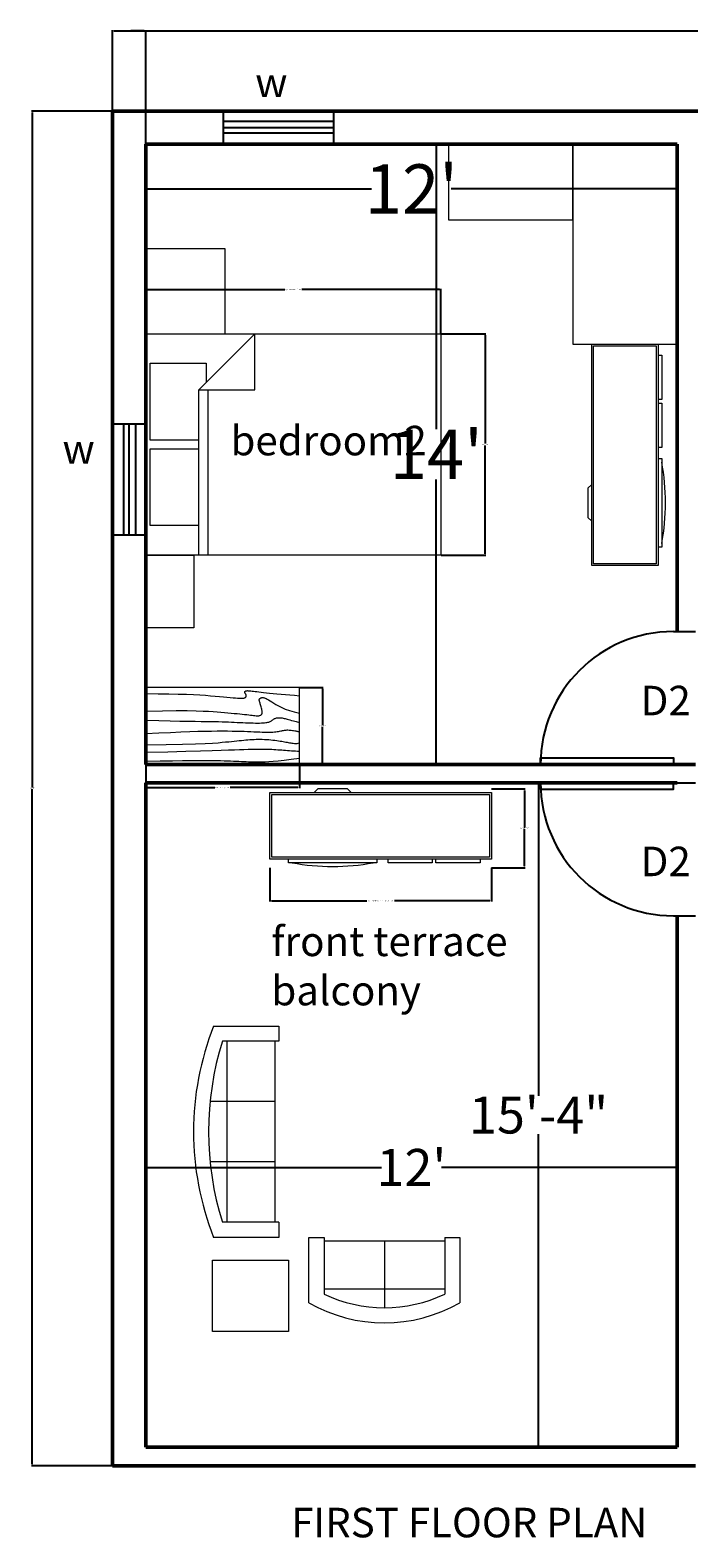
# Model space of a CAD drawing. Units: inches. Extents: x -10 to 557, y -66 to 886.
# Tile 4 of 6: x 31 to 210, y 478 to 886. Entities that reach past the tile are written whole.
import ezdxf

# ---------------------------------------------------------------- set-up
doc = ezdxf.new("R2010")
doc.units = ezdxf.units.IN
doc.header["$MEASUREMENT"] = 0
for name, color, linetype, lineweight in [('A-ANNO-DIMS', 2, 'Continuous', 18), ('A-ANNO-TEXT', 7, 'Continuous', 18), ('A-AREA-IDEN', 7, 'Continuous', 25), ('A-DOOR', 4, 'Continuous', 25), ('A-FURN', 8, 'Continuous', 18), ('A-GLAZ', 4, 'Continuous', 25), ('A-WALL', 7, 'Continuous', 50)]:
    doc.layers.add(name, color=color, linetype=linetype, lineweight=lineweight)
doc.styles.get("Standard").update_dxf_attribs({"font": 'arial.ttf'})
doc.dimstyles.get("Standard").update_dxf_attribs({"dimtxt": 0.3, "dimasz": 0.4, "dimexe": 0.18, "dimexo": 0.0625, "dimgap": 0.09, "dimtad": 0, "dimtih": 1, "dimtoh": 1, "dimdec": 0, "dimrnd": 8, "dimzin": 0, "dimdsep": 46, "dimlunit": 3, "dimtxsty": 'Standard', "dimcen": 0.09, "dimadec": 0, "dimazin": 0, "dimtfac": 1, "dimtdec": 0, "dimtofl": 0, "dimtmove": 0, "dimatfit": 3, "dimfxl": 1, "dimtolj": 1, "dimtzin": 0, "dimarcsym": 0})

# ---------------------------------------------------------------- blocks, each defined once
blk = doc.blocks.new('*U2')
for p, q in [((0, 0), (0, -6)), ((36, 0), (36, -6))]:
    blk.add_line(p, q)
blk.add_lwpolyline([(0, 0), (0, 36), (1.75, 36), (1.75, 0)], close=True)
blk.add_arc((0, 0), 36, 0, 90)
blk = doc.blocks.new('*U5')
for p, q in [((0, 0), (0, -6)), ((-36, 0), (-36, -6))]:
    blk.add_line(p, q)
blk.add_lwpolyline([(0, 0), (0, 36), (-1.75, 36), (-1.75, 0)], close=True)
blk.add_arc((0, 0), 36, 90, 180)
blk = doc.blocks.new('Entertainment Center')
for p, q in [((-4, 0), (-5, -1)), ((4, 0), (-4, 0)), ((5, -1), (4, 0)), ((-17, -19), (-17, -1)), ((-17, -1), (43, -1)), ((-16.5, -18.5), (-16.5, -1.5)), ((-16.5, -1.5), (42.5, -1.5)), ((42.5, -1.5), (42.5, -18.5)), ((43, -1), (43, -19)), ((43, -19), (-17, -19)), ((42.5, -18.5), (-16.5, -18.5)), ((-12, -20), (-12, -19)), ((12, -20), (-12, -20)), ((12, -19), (12, -20)), ((15, -20), (15, -19)), ((27, -20), (15, -20)), ((27, -19), (27, -20)), ((28, -20), (28, -19)), ((40, -20), (28, -20)), ((40, -19), (40, -20))]:
    blk.add_line(p, q)
blk.add_arc((0, 40), 61, 259.6111, 280.3889)
blk = doc.blocks.new('Sofa - Roundback 7 ft.')
for p, q in [((-36.000027, -34), (-36.000027, -11.4696)), ((-12.00002, -32.4421), (-12.00003, -6.5971)), ((11.99997, -32.4421), (11.99998, -6.5971)), ((35.99998, -34), (35.99998, -11.4696)), ((-35.999844, -13.3819), (35.9998, -13.3819)), ((-36.000027, -32.4421), (35.99998, -32.4421))]:
    blk.add_line(p, q)
for points in [[(-36.000027, -34), (-42.000027, -34), (-42.000027, -8)], [(41.99998, -8), (41.99998, -34), (35.99998, -34)]]:
    blk.add_lwpolyline(points)
for centre, radius, start, end in [((0, -114.25), 114.25, 68.43141, 111.5686), ((-0.00001, -127.1968), 121.1968, 72.72033, 107.2797)]:
    blk.add_arc(centre, radius, start, end)
blk = doc.blocks.new('Sofa - Roundback Loveseat 5 ft.')
for p, q in [((-24, -33.99998), (-24, -11.46958)), ((0, -32.44198), (0, -5.99998)), ((24.00004, -33.99998), (24.00004, -11.46958)), ((-23.9998, -13.38178), (23.99986, -13.38178)), ((-24, -32.44198), (24.00004, -32.44198))]:
    blk.add_line(p, q)
for points in [[(-24, -33.99998), (-30, -33.99998), (-30, -7.99998)], [(30.00004, -7.99998), (30.00004, -33.99998), (24.00004, -33.99998)]]:
    blk.add_lwpolyline(points)
for centre, radius, start, end in [((0, -60.24998), 60.24998, 60.13715, 119.8628), ((0, -61.38438), 55.38444, 64.32083, 115.6792)]:
    blk.add_arc(centre, radius, start, end)
blk = doc.blocks.new('Bed - Queen')
for p, q in [((0, -80.00003), (0, 0)), ((0, 0), (59.99999, 0)), ((59.99999, 0), (59.99999, -80.00003)), ((7.99999, -1.2), (28.79998, -1.2)), ((7.99999, -14.4), (7.99999, -1.2)), ((28.79998, -1.2), (28.79998, -14.4)), ((31.19999, -1.2), (51.99999, -1.2)), ((31.19999, -14.4), (31.19999, -1.2)), ((51.99999, -1.2), (51.99999, -16.4)), ((0, -14.4), (44.8, -14.4)), ((59.99999, -29.6), (44.8, -14.4)), ((44.8, -14.4), (44.8, -29.6)), ((44.8, -16.8), (0, -16.8)), ((51.99999, -16.4), (46.79936, -16.4)), ((44.8, -29.6), (59.99999, -29.6)), ((59.99999, -80.00003), (0, -80.00003))]:
    blk.add_line(p, q)
blk = doc.blocks.new('Table - Rectangular Woodgrain 60 x 30 in.')
for p, q in [((0, 0), (0, -30)), ((60, 0), (0, 0)), ((60, -30), (60, 0)), ((0, -30), (60, -30))]:
    blk.add_line(p, q)
for points in [[(0, -2.4), (4.8155, -2.418), (9.0302, -2.4688), (12.709, -2.5477), (15.9167, -2.65), (18.7181, -2.7711), (21.1781, -2.9063), (23.3616, -3.0508), (25.3333, -3.2), (27.1477, -3.3495), (28.8172, -3.4958), (30.3437, -3.636), (31.7291, -3.7667), (32.9756, -3.8849), (34.0849, -3.9875), (35.059, -4.0714), (35.9, -4.1334), (36.6114, -4.1711), (37.2041, -4.1854), (37.6906, -4.1779), (38.0833, -4.15), (38.3948, -4.1034), (38.6375, -4.0396), (38.8239, -3.9602), (38.9666, -3.8667), (39.0764, -3.7608), (39.1573, -3.6448), (39.2116, -3.521), (39.2416, -3.3917), (39.2498, -3.2593), (39.2385, -3.1261), (39.21, -2.9944), (39.1666, -2.8667), (39.111, -2.7447), (39.0468, -2.6281), (38.978, -2.5163), (38.9083, -2.4083), (38.8418, -2.3035), (38.7823, -2.201), (38.7337, -2.1001), (38.7, -2), (38.6844, -1.9003), (38.6875, -1.8021), (38.7094, -1.707), (38.75, -1.6167), (38.8094, -1.5326), (38.8875, -1.4563), (38.9844, -1.3893), (39.1, -1.3333), (39.2351, -1.2896), (39.3937, -1.2583), (39.5804, -1.2396), (39.8, -1.2333), (40.057, -1.2396), (40.3562, -1.2583), (40.7023, -1.2896), (41.1, -1.3333), (41.5547, -1.3895), (42.0755, -1.4573), (42.6721, -1.5361), (43.3542, -1.625), (44.1316, -1.7233), (45.014, -1.8302), (46.0114, -1.9449), (47.1333, -2.0667), (48.3862, -2.1947), (49.7625, -2.3281), (51.2513, -2.4663), (52.8416, -2.6083), (54.5226, -2.7535), (56.2833, -2.9011), (58.1127, -3.0501), (60, -3.2)], [(0, -9.2), (6.5759, -9.0858), (11.9385, -9.0365), (16.2527, -9.0418), (19.6833, -9.0917), (22.3952, -9.1759), (24.5531, -9.2844), (26.322, -9.4069), (27.8666, -9.5333), (29.3241, -9.6553), (30.7203, -9.7719), (32.0532, -9.8837), (33.3208, -9.9917), (34.5213, -10.0965), (35.6526, -10.199), (36.7128, -10.2999), (37.7, -10.4), (38.6129, -10.4996), (39.4531, -10.5969), (40.223, -10.6895), (40.925, -10.775), (41.5613, -10.8512), (42.1344, -10.9156), (42.6465, -10.966), (43.1, -11), (43.4976, -11.0158), (43.8437, -11.0136), (44.143, -10.9942), (44.4, -10.9583), (44.6195, -10.9069), (44.8062, -10.8406), (44.9648, -10.7603), (45.1, -10.6667), (45.2155, -10.5598), (45.3114, -10.4365), (45.3871, -10.2929), (45.4416, -10.125), (45.4743, -9.929), (45.4844, -9.7011), (45.4709, -9.4371), (45.4333, -9.1333), (45.3716, -8.7883), (45.2896, -8.4104), (45.1919, -8.0107), (45.0833, -7.6), (44.9685, -7.1893), (44.8521, -6.7896), (44.7388, -6.4117), (44.6333, -6.0667), (44.54, -5.7628), (44.4614, -5.4979), (44.4001, -5.2675), (44.3583, -5.0667), (44.3384, -4.8909), (44.3427, -4.7354), (44.3736, -4.5956), (44.4333, -4.4667), (44.5236, -4.3453), (44.6427, -4.2333), (44.7884, -4.1339), (44.9583, -4.05), (45.1501, -3.9849), (45.3614, -3.9417), (45.59, -3.9234), (45.8333, -3.9333), (46.0915, -3.9749), (46.3734, -4.0531), (46.6906, -4.1736), (47.0542, -4.3417), (47.4756, -4.5629), (47.9661, -4.8427), (48.5372, -5.1866), (49.2, -5.6), (49.9676, -6.0844), (50.8594, -6.625), (51.8965, -7.2031), (53.1, -7.8), (54.491, -8.3969), (56.0906, -8.975), (57.9199, -9.5156), (60, -10)], [(0, -12.8), (5.1847, -12.9322), (9.6213, -13.0323), (13.3963, -13.1059), (16.5958, -13.1583), (19.3063, -13.1952), (21.614, -13.2219), (23.6054, -13.2439), (25.3666, -13.2667), (26.9728, -13.2947), (28.4531, -13.3281), (29.8256, -13.3663), (31.1083, -13.4083), (32.3191, -13.4535), (33.476, -13.501), (34.597, -13.5501), (35.7, -13.6), (36.7984, -13.6497), (37.8875, -13.6979), (38.9578, -13.743), (40, -13.7833), (41.0047, -13.8174), (41.9625, -13.8438), (42.864, -13.8607), (43.7, -13.8667), (44.4631, -13.8604), (45.1552, -13.8417), (45.7801, -13.8104), (46.3416, -13.7667), (46.8439, -13.7104), (47.2906, -13.6417), (47.6858, -13.5604), (48.0333, -13.4667), (48.3375, -13.3608), (48.6042, -13.2448), (48.8396, -13.121), (49.05, -12.9917), (49.2417, -12.8593), (49.4208, -12.7261), (49.5937, -12.5944), (49.7667, -12.4667), (49.9452, -12.3451), (50.1323, -12.2313), (50.3303, -12.1268), (50.5416, -12.0333), (50.7686, -11.9524), (51.0135, -11.8854), (51.2788, -11.8341), (51.5666, -11.8), (51.8785, -11.7843), (52.2116, -11.7865), (52.562, -11.8059), (52.926, -11.8417), (53.2998, -11.8931), (53.6795, -11.9594), (54.0614, -12.0397), (54.4416, -12.1333), (54.8223, -12.2401), (55.2293, -12.3625), (55.6942, -12.5037), (56.2489, -12.6667), (56.9251, -12.8547), (57.7545, -13.0708), (58.7689, -13.3182), (60, -13.6)], [(0, -18), (5.124, -17.7273), (9.6609, -17.5057), (13.6705, -17.3303), (17.2125, -17.1958), (20.3467, -17.0973), (23.1328, -17.0297), (25.6307, -16.9878), (27.9, -16.9667), (29.9928, -16.9617), (31.9302, -16.9703), (33.7254, -16.9907), (35.3917, -17.0208), (36.9423, -17.0588), (38.3906, -17.1026), (39.7499, -17.1503), (41.0333, -17.2), (42.2519, -17.2496), (43.4073, -17.2969), (44.4986, -17.3395), (45.525, -17.375), (46.4858, -17.4012), (47.3802, -17.4156), (48.2074, -17.416), (48.9667, -17.4), (49.6583, -17.3662), (50.2872, -17.3167), (50.8595, -17.2547), (51.3812, -17.1833), (51.8584, -17.1057), (52.2971, -17.025), (52.7034, -16.9443), (53.0833, -16.8667), (53.443, -16.7951), (53.789, -16.7313), (54.128, -16.6768), (54.4666, -16.6334), (54.8115, -16.6024), (55.1693, -16.5854), (55.5465, -16.5841), (55.95, -16.6), (56.3828, -16.6337), (56.8346, -16.6823), (57.2915, -16.7418), (57.7396, -16.8084), (58.165, -16.878), (58.5539, -16.9469), (58.8924, -17.0111), (59.1666, -17.0667), (59.3679, -17.1107), (59.5078, -17.1438), (59.6032, -17.1675), (59.6708, -17.1833), (59.7275, -17.193), (59.7901, -17.1979), (59.8753, -17.1998), (60, -17.2)], [(0, -22.4), (8.0098, -22.2501), (14.4094, -22.1011), (19.4168, -21.9535), (23.25, -21.8083), (26.1269, -21.6663), (28.2656, -21.5281), (29.884, -21.3947), (31.2, -21.2667), (32.3967, -21.1448), (33.5172, -21.0292), (34.5697, -20.9198), (35.5625, -20.8167), (36.5037, -20.7198), (37.4015, -20.6292), (38.2642, -20.5448), (39.1, -20.4667), (39.9164, -20.3951), (40.7187, -20.3313), (41.5117, -20.2768), (42.3, -20.2333), (43.0883, -20.2024), (43.8812, -20.1854), (44.6836, -20.1841), (45.5, -20.2), (46.3328, -20.234), (47.1747, -20.2844), (48.0163, -20.3488), (48.8479, -20.425), (49.66, -20.5106), (50.4429, -20.6031), (51.1872, -20.7004), (51.8833, -20.8), (52.5246, -20.8999), (53.1166, -20.9995), (53.6681, -21.0983), (54.1875, -21.1958), (54.6834, -21.2919), (55.1646, -21.3859), (55.6394, -21.4777), (56.1167, -21.5667), (56.6028, -21.6515), (57.0961, -21.7266), (57.5929, -21.7852), (58.0896, -21.8208), (58.5823, -21.8268), (59.0674, -21.7964), (59.5412, -21.723), (60, -21.6)], [(0, -25.2), (8.6355, -25.0504), (15.7026, -24.9031), (21.4049, -24.7606), (25.9458, -24.625), (29.529, -24.4988), (32.3578, -24.3844), (34.6359, -24.284), (36.5667, -24.2), (38.3213, -24.1341), (39.9417, -24.0854), (41.437, -24.0523), (42.8167, -24.0333), (44.0901, -24.0268), (45.2667, -24.0313), (46.3557, -24.0451), (47.3667, -24.0667), (48.309, -24.0947), (49.1928, -24.1287), (50.0284, -24.168), (50.826, -24.2125), (51.5959, -24.2617), (52.3483, -24.3151), (53.0935, -24.3725), (53.8417, -24.4334), (54.6009, -24.497), (55.3699, -24.561), (56.1454, -24.6226), (56.9239, -24.6792), (57.7021, -24.7279), (58.4764, -24.7662), (59.2435, -24.7911), (60, -24.8)], [(0, -28.8), (5.6867, -28.6681), (10.45, -28.5698), (14.407, -28.5012), (17.675, -28.4584), (20.3711, -28.4374), (22.6125, -28.4344), (24.5164, -28.4455), (26.2, -28.4667), (27.762, -28.4947), (29.2276, -28.5281), (30.6033, -28.5663), (31.8958, -28.6084), (33.1118, -28.6535), (34.2578, -28.7011), (35.3405, -28.7501), (36.3666, -28.8), (37.3443, -28.8497), (38.288, -28.8974), (39.2137, -28.9412), (40.1375, -28.9792), (41.0753, -29.0093), (42.0432, -29.0297), (43.0572, -29.0384), (44.1333, -29.0333), (45.2936, -29.0114), (46.5843, -28.9641), (48.0579, -28.8816), (49.7666, -28.7542), (51.7629, -28.5721), (54.0989, -28.3255), (56.8272, -28.0048), (60, -27.6)]]:
    blk.add_lwpolyline(points)
blk = doc.blocks.new('*D15')
at = {"layer": 'A-ANNO-DIMS', "color": 0, "lineweight": -2, "transparency": 16777216}
for p, q in [((147.17, 855.2), (141.22, 855.2)), ((141.4, 854.8), (141.4, 777.98)), ((141.4, 687.6), (141.4, 764.41)), ((147.17, 687.2), (141.22, 687.2))]:
    blk.add_line(p, q, dxfattribs=at)
at = {"layer": 'A-ANNO-DIMS', "color": 0, "transparency": 16777216}
for points in [[(141.33, 854.8), (141.46, 854.8), (141.4, 855.2)], [(141.33, 687.6), (141.46, 687.6), (141.4, 687.2)]]:
    blk.add_solid(points, dxfattribs=at)
at = {"layer": 'Defpoints', "color": 0, "transparency": 16777216}
for p in [(147.23, 855.2), (141.4, 687.2), (147.23, 687.2)]:
    blk.add_point(p, dxfattribs=at)
at = {"layer": 'A-ANNO-DIMS', "color": 0, "transparency": 16777216, "insert": (141.4, 771.2), "char_height": 0.3, "attachment_point": 5}
blk.add_mtext("\\A1;{\\H44.44444x;14'}", dxfattribs=at)
blk = doc.blocks.new('*D16')
at = {"layer": 'A-ANNO-DIMS', "color": 0, "lineweight": -2, "transparency": 16777216}
for p, q in [((62.66, 855.13), (62.66, 842.91)), ((206.66, 855.13), (206.66, 842.91)), ((63.06, 843.09), (123.89, 843.09)), ((206.26, 843.09), (145.44, 843.09))]:
    blk.add_line(p, q, dxfattribs=at)
at = {"layer": 'A-ANNO-DIMS', "color": 0, "transparency": 16777216}
for points in [[(63.06, 843.16), (63.06, 843.03), (62.66, 843.09)], [(206.26, 843.16), (206.26, 843.03), (206.66, 843.09)]]:
    blk.add_solid(points, dxfattribs=at)
at = {"layer": 'Defpoints', "color": 0, "transparency": 16777216}
for p in [(62.66, 855.2), (206.66, 855.2), (206.66, 843.09)]:
    blk.add_point(p, dxfattribs=at)
at = {"layer": 'A-ANNO-DIMS', "color": 0, "transparency": 16777216, "insert": (134.66, 843.09), "char_height": 0.3, "attachment_point": 5}
blk.add_mtext("\\A1;{\\H44.44444x;12'}", dxfattribs=at)
blk = doc.blocks.new('*D27')
at = {"layer": 'A-ANNO-DIMS', "color": 0, "lineweight": -2, "transparency": 16777216}
for p, q in [((164.05, 682.2), (169.3, 682.2)), ((169.12, 681.8), (169.12, 597.39)), ((169.12, 502.6), (169.12, 587)), ((164.05, 502.2), (169.3, 502.2))]:
    blk.add_line(p, q, dxfattribs=at)
at = {"layer": 'A-ANNO-DIMS', "color": 0, "transparency": 16777216}
for points in [[(169.06, 681.8), (169.19, 681.8), (169.12, 682.2)], [(169.06, 502.6), (169.19, 502.6), (169.12, 502.2)]]:
    blk.add_solid(points, dxfattribs=at)
at = {"layer": 'Defpoints', "color": 0, "transparency": 16777216}
for p in [(163.99, 682.2), (163.99, 502.2), (169.12, 502.2)]:
    blk.add_point(p, dxfattribs=at)
at = {"layer": 'A-ANNO-DIMS', "color": 0, "transparency": 16777216, "insert": (169.12, 592.2), "char_height": 0.3, "attachment_point": 5}
blk.add_mtext('\\A1;{\\H33.33333x;15\'-4"}', dxfattribs=at)
blk = doc.blocks.new('*D28')
at = {"layer": 'A-ANNO-DIMS', "color": 0, "lineweight": -2, "transparency": 16777216}
for p, q in [((62.66, 587.17), (62.66, 577.84)), ((206.66, 587.17), (206.66, 577.84)), ((63.06, 578.02), (126.56, 578.02)), ((206.26, 578.02), (142.77, 578.02))]:
    blk.add_line(p, q, dxfattribs=at)
at = {"layer": 'A-ANNO-DIMS', "color": 0, "transparency": 16777216}
for points in [[(63.06, 578.09), (63.06, 577.96), (62.66, 578.02)], [(206.26, 578.09), (206.26, 577.96), (206.66, 578.02)]]:
    blk.add_solid(points, dxfattribs=at)
at = {"layer": 'Defpoints', "color": 0, "transparency": 16777216}
for p in [(62.66, 587.23), (206.66, 587.23), (206.66, 578.02)]:
    blk.add_point(p, dxfattribs=at)
at = {"layer": 'A-ANNO-DIMS', "color": 0, "transparency": 16777216, "insert": (134.66, 578.02), "char_height": 0.3, "attachment_point": 5}
blk.add_mtext("\\A1;{\\H33.33333x;12'}", dxfattribs=at)
blk = doc.blocks.new('WIN-900')
for p, q in [((0, 6.25), (30, 6.25)), ((0, 4.5), (30, 4.5)), ((0, 3.05), (30, 3.05))]:
    blk.add_line(p, q)
blk.add_lwpolyline([(0, 9), (0, 0), (30, 0), (30, 9)], close=True)
blk = doc.blocks.new('*D55')
at = {"layer": 'A-ANNO-DIMS', "color": 0, "lineweight": -2, "ltscale": 2, "transparency": 16777216}
for p, q in [((62.65, 687.14), (62.65, 680.77)), ((104.3, 687.14), (104.3, 680.77)), ((63.05, 680.95), (81.4, 680.95)), ((103.9, 680.95), (85.55, 680.95))]:
    blk.add_line(p, q, dxfattribs=at)
at = {"layer": 'A-ANNO-DIMS', "color": 0, "ltscale": 2, "transparency": 16777216}
for points in [[(63.05, 681.02), (63.05, 680.89), (62.65, 680.95)], [(103.9, 681.02), (103.9, 680.89), (104.3, 680.95)]]:
    blk.add_solid(points, dxfattribs=at)
at = {"layer": 'Defpoints', "color": 0, "ltscale": 2, "transparency": 16777216}
for p in [(62.65, 687.2), (104.3, 687.2), (104.3, 680.95)]:
    blk.add_point(p, dxfattribs=at)
at = {"layer": 'A-ANNO-DIMS', "color": 0, "ltscale": 2, "transparency": 16777216, "insert": (83.47, 680.95), "char_height": 0.3, "attachment_point": 5}
blk.add_mtext('\\A1;TABLE 3\'-5 1/2" TYP.', dxfattribs=at)
blk = doc.blocks.new('*D56')
at = {"layer": 'A-ANNO-DIMS', "color": 0, "lineweight": -2, "ltscale": 2, "transparency": 16777216}
for p, q in [((104.37, 708.03), (110.73, 708.03)), ((110.55, 707.63), (110.55, 697.86)), ((110.55, 687.6), (110.55, 697.37)), ((104.37, 687.2), (110.73, 687.2))]:
    blk.add_line(p, q, dxfattribs=at)
at = {"layer": 'A-ANNO-DIMS', "color": 0, "ltscale": 2, "transparency": 16777216}
for points in [[(110.49, 707.63), (110.62, 707.63), (110.55, 708.03)], [(110.49, 687.6), (110.62, 687.6), (110.55, 687.2)]]:
    blk.add_solid(points, dxfattribs=at)
at = {"layer": 'Defpoints', "color": 0, "ltscale": 2, "transparency": 16777216}
for p in [(104.3, 708.03), (110.55, 708.03), (104.3, 687.2)]:
    blk.add_point(p, dxfattribs=at)
at = {"layer": 'A-ANNO-DIMS', "color": 0, "ltscale": 2, "transparency": 16777216, "insert": (110.55, 697.62), "char_height": 0.3, "attachment_point": 5}
blk.add_mtext('\\A1;1\'-9" TYP.', dxfattribs=at)
blk = doc.blocks.new('*D59')
at = {"layer": 'A-ANNO-DIMS', "color": 0, "lineweight": -2, "ltscale": 2, "transparency": 16777216}
for p, q in [((96.32, 659.15), (96.32, 650.03)), ((156.32, 659.15), (156.32, 650.03)), ((96.72, 650.21), (122.56, 650.21)), ((155.92, 650.21), (130.07, 650.21))]:
    blk.add_line(p, q, dxfattribs=at)
at = {"layer": 'A-ANNO-DIMS', "color": 0, "ltscale": 2, "transparency": 16777216}
for points in [[(96.72, 650.28), (96.72, 650.14), (96.32, 650.21)], [(155.92, 650.28), (155.92, 650.14), (156.32, 650.21)]]:
    blk.add_solid(points, dxfattribs=at)
at = {"layer": 'Defpoints', "color": 0, "ltscale": 2, "transparency": 16777216}
for p in [(96.32, 659.21), (156.32, 659.21), (156.32, 650.21)]:
    blk.add_point(p, dxfattribs=at)
at = {"layer": 'A-ANNO-DIMS', "color": 0, "ltscale": 2, "transparency": 16777216, "insert": (126.32, 650.21), "char_height": 0.3, "attachment_point": 5}
blk.add_mtext('\\A1;ENTERTAINMENT CENTER 5\'-0" TYP.', dxfattribs=at)
blk = doc.blocks.new('*D60')
at = {"layer": 'A-ANNO-DIMS', "color": 0, "lineweight": -2, "ltscale": 2, "transparency": 16777216}
for p, q in [((156.38, 680.54), (165.5, 680.54)), ((165.32, 680.14), (165.32, 670.12)), ((165.32, 659.61), (165.32, 669.63)), ((156.38, 659.21), (165.5, 659.21))]:
    blk.add_line(p, q, dxfattribs=at)
at = {"layer": 'A-ANNO-DIMS', "color": 0, "ltscale": 2, "transparency": 16777216}
for points in [[(165.25, 680.14), (165.39, 680.14), (165.32, 680.54)], [(165.25, 659.61), (165.39, 659.61), (165.32, 659.21)]]:
    blk.add_solid(points, dxfattribs=at)
at = {"layer": 'Defpoints', "color": 0, "ltscale": 2, "transparency": 16777216}
for p in [(156.32, 680.54), (165.32, 680.54), (156.32, 659.21)]:
    blk.add_point(p, dxfattribs=at)
at = {"layer": 'A-ANNO-DIMS', "color": 0, "ltscale": 2, "transparency": 16777216, "insert": (165.32, 669.88), "char_height": 0.3, "attachment_point": 5}
blk.add_mtext('\\A1;1\'-9 1/2" TYP.', dxfattribs=at)
blk = doc.blocks.new('*D65')
at = {"layer": 'A-ANNO-DIMS', "color": 0, "lineweight": -2, "ltscale": 2, "transparency": 16777216}
for p, q in [((62.66, 803.93), (62.66, 816.05)), ((63.06, 815.87), (100.37, 815.87)), ((142.26, 815.87), (104.96, 815.87)), ((142.66, 803.93), (142.66, 816.05))]:
    blk.add_line(p, q, dxfattribs=at)
at = {"layer": 'A-ANNO-DIMS', "color": 0, "ltscale": 2, "transparency": 16777216}
for points in [[(63.06, 815.94), (63.06, 815.8), (62.66, 815.87)], [(142.26, 815.94), (142.26, 815.8), (142.66, 815.87)]]:
    blk.add_solid(points, dxfattribs=at)
at = {"layer": 'Defpoints', "color": 0, "ltscale": 2, "transparency": 16777216}
for p in [(62.66, 815.87), (62.66, 803.87), (142.66, 803.87)]:
    blk.add_point(p, dxfattribs=at)
at = {"layer": 'A-ANNO-DIMS', "color": 0, "ltscale": 2, "transparency": 16777216, "insert": (102.66, 815.87), "char_height": 0.3, "attachment_point": 5}
blk.add_mtext('\\A1;QUEEN BED 6\'-8" TYP.', dxfattribs=at)
blk = doc.blocks.new('*D66')
at = {"layer": 'A-ANNO-DIMS', "color": 0, "lineweight": -2, "ltscale": 2, "transparency": 16777216}
for p, q in [((142.73, 803.87), (154.84, 803.87)), ((154.66, 803.47), (154.66, 774.11)), ((154.66, 744.27), (154.66, 773.63)), ((142.73, 743.87), (154.84, 743.87))]:
    blk.add_line(p, q, dxfattribs=at)
at = {"layer": 'A-ANNO-DIMS', "color": 0, "ltscale": 2, "transparency": 16777216}
for points in [[(154.6, 803.47), (154.73, 803.47), (154.66, 803.87)], [(154.6, 744.27), (154.73, 744.27), (154.66, 743.87)]]:
    blk.add_solid(points, dxfattribs=at)
at = {"layer": 'Defpoints', "color": 0, "ltscale": 2, "transparency": 16777216}
for p in [(142.66, 803.87), (154.66, 803.87), (142.66, 743.87)]:
    blk.add_point(p, dxfattribs=at)
at = {"layer": 'A-ANNO-DIMS', "color": 0, "ltscale": 2, "transparency": 16777216, "insert": (154.66, 773.87), "char_height": 0.3, "attachment_point": 5}
blk.add_mtext('\\A1;5\'-0" TYP.', dxfattribs=at)
blk = doc.blocks.new('*D79')
at = {"layer": 'A-ANNO-DIMS', "color": 0, "lineweight": -2, "ltscale": 2, "transparency": 16777216}
for p, q in [((53.66, 864.26), (53.66, 886.09)), ((54.06, 885.91), (57.67, 885.91)), ((62.26, 885.91), (58.65, 885.91)), ((62.66, 855.26), (62.66, 886.09))]:
    blk.add_line(p, q, dxfattribs=at)
at = {"layer": 'A-ANNO-DIMS', "color": 0, "ltscale": 2, "transparency": 16777216}
for points in [[(54.06, 885.97), (54.06, 885.84), (53.66, 885.91)], [(62.26, 885.97), (62.26, 885.84), (62.66, 885.91)]]:
    blk.add_solid(points, dxfattribs=at)
at = {"layer": 'Defpoints', "color": 0, "ltscale": 2, "transparency": 16777216}
for p in [(62.66, 885.91), (53.66, 864.2), (62.66, 855.2)]:
    blk.add_point(p, dxfattribs=at)
at = {"layer": 'A-ANNO-DIMS', "color": 0, "ltscale": 2, "transparency": 16777216, "insert": (58.16, 885.91), "char_height": 0.3, "attachment_point": 5}
blk.add_mtext('\\A1;0\'-9"', dxfattribs=at)
blk = doc.blocks.new('*D81')
at = {"layer": 'A-ANNO-DIMS', "color": 0, "lineweight": -2, "ltscale": 2, "transparency": 16777216}
for p, q in [((53.66, 864.26), (53.66, 886.09)), ((54.06, 885.91), (259.56, 885.91)), ((466.26, 885.91), (260.77, 885.91)), ((466.66, 807.26), (466.66, 886.09))]:
    blk.add_line(p, q, dxfattribs=at)
at = {"layer": 'A-ANNO-DIMS', "color": 0, "ltscale": 2, "transparency": 16777216}
for points in [[(54.06, 885.97), (54.06, 885.84), (53.66, 885.91)], [(466.26, 885.97), (466.26, 885.84), (466.66, 885.91)]]:
    blk.add_solid(points, dxfattribs=at)
at = {"layer": 'Defpoints', "color": 0, "ltscale": 2, "transparency": 16777216}
for p in [(466.66, 885.91), (53.66, 864.2), (466.66, 807.2)]:
    blk.add_point(p, dxfattribs=at)
at = {"layer": 'A-ANNO-DIMS', "color": 0, "ltscale": 2, "transparency": 16777216, "insert": (260.16, 885.91), "char_height": 0.3, "attachment_point": 5}
blk.add_mtext('\\A1;34\'-5"', dxfattribs=at)
blk = doc.blocks.new('*D82')
at = {"layer": 'A-ANNO-DIMS', "color": 0, "lineweight": -2, "ltscale": 2, "transparency": 16777216}
for p, q in [((53.6, 864.2), (31.73, 864.2)), ((31.91, 863.8), (31.91, 680.94)), ((31.91, 497.6), (31.91, 680.45)), ((53.6, 497.2), (31.73, 497.2))]:
    blk.add_line(p, q, dxfattribs=at)
at = {"layer": 'A-ANNO-DIMS', "color": 0, "ltscale": 2, "transparency": 16777216}
for points in [[(31.84, 863.8), (31.98, 863.8), (31.91, 864.2)], [(31.84, 497.6), (31.98, 497.6), (31.91, 497.2)]]:
    blk.add_solid(points, dxfattribs=at)
at = {"layer": 'Defpoints', "color": 0, "ltscale": 2, "transparency": 16777216}
for p in [(31.91, 864.2), (53.66, 864.2), (53.66, 497.2)]:
    blk.add_point(p, dxfattribs=at)
at = {"layer": 'A-ANNO-DIMS', "color": 0, "ltscale": 2, "transparency": 16777216, "insert": (31.91, 680.7), "char_height": 0.3, "attachment_point": 5}
blk.add_mtext('\\A1;30\'-7"', dxfattribs=at)

msp = doc.modelspace()

# ---------------------------------------------------------------- linework, layer by layer
at = {"layer": 'A-FURN'}
for points in [[(178.43, 855.2), (144.75, 855.2), (144.75, 834.7), (178.43, 834.7)], [(206.66, 855.2), (178.43, 855.2), (178.43, 801.06), (206.66, 801.06)], [(62.66, 803.87), (84.17, 803.87), (84.17, 826.82), (62.66, 826.82)], [(62.66, 743.87), (75.68, 743.87), (75.68, 724.16), (62.66, 724.16)], [(80.75, 552.87), (101.31, 552.87), (101.31, 533.61), (80.75, 533.61)]]:
    msp.add_lwpolyline(points, close=True, dxfattribs=at)
at = {"layer": 'A-WALL'}
for p, q in [((53.66, 864.2), (413.66, 864.2)), ((53.66, 497.2), (53.66, 864.2)), ((62.66, 855.2), (206.66, 855.2)), ((62.66, 687.2), (62.66, 855.2)), ((206.66, 723.2), (206.66, 855.2)), ((62.66, 687.2), (206.66, 687.2)), ((206.66, 687.2), (211.66, 687.2)), ((62.66, 502.2), (62.66, 682.2)), ((62.66, 682.2), (206.66, 682.2)), ((206.66, 502.2), (206.66, 646.2)), ((62.66, 502.2), (206.66, 502.2)), ((53.66, 497.2), (211.66, 497.2))]:
    msp.add_line(p, q, dxfattribs=at)

# ---------------------------------------------------------------- block references
at = {"layer": 'A-DOOR', "rotation": 90}
for name, p in [('*U2', (205.66, 687.2)), ('*U5', (205.66, 682.2))]:
    msp.add_blockref(name, p, dxfattribs=at)
at = {"layer": 'A-FURN', "rotation": 90}
for name, p in [('Bed - Queen', (62.66, 743.87)), ('Entertainment Center', (182.51, 758.06))]:
    msp.add_blockref(name, p, dxfattribs=at)
at = {"layer": 'A-FURN', "xscale": 0.6942880543039835, "yscale": 0.6942880543039835, "zscale": 0.6942880543039835}
msp.add_blockref('Table - Rectangular Woodgrain 60 x 30 in.', (62.65, 708.03), dxfattribs=at)
msp.add_blockref('Table - Rectangular Woodgrain 60 x 30 in.', (62.65, 708.03), dxfattribs=at)
msp.add_blockref('Table - Rectangular Woodgrain 60 x 30 in.', (62.65, 708.03), dxfattribs=at)
msp.add_blockref('Table - Rectangular Woodgrain 60 x 30 in.', (62.65, 708.03), dxfattribs=at)
at = {"layer": 'A-FURN'}
msp.add_blockref('Entertainment Center', (113.32, 680.54), dxfattribs=at)
at = {"layer": 'A-FURN', "xscale": 0.6812959275706195, "yscale": 0.6812959275706195, "zscale": 0.6812959275706195}
for name, p, rotation in [('Sofa - Roundback 7 ft.', (75.61, 587.69), 90), ('Sofa - Roundback Loveseat 5 ft.', (127.33, 535.91), 180)]:
    msp.add_blockref(name, p, dxfattribs=dict(at, rotation=rotation))
at = {"layer": 'A-GLAZ'}
msp.add_blockref('WIN-900', (83.63, 855.21), dxfattribs=at)
at = {"layer": 'A-GLAZ', "rotation": 270.0000000000005}
msp.add_blockref('WIN-900', (53.61, 779.41), dxfattribs=at)

# ---------------------------------------------------------------- texts
at = {"layer": 'A-ANNO-TEXT', "char_height": 8, "attachment_point": 1}
for s, width, heights, insert in [('w', 13.506, [0], (92.33, 875.95)), ('w', 13.506, [0], (40.1, 776.65)), ('D2', 13.506, [0], (196.79, 708.49)), ('D2', 13.506, [0], (196.79, 664.91)), ('FIRST FLOOR PLAN', 271.5145, [0.207], (102.06, 485.81))]:
    msp.add_mtext_dynamic_manual_height_columns(s, width=width, gutter_width=1, heights=heights, dxfattribs=dict(at, insert=insert))
at = {"layer": 'A-AREA-IDEN', "char_height": 8, "attachment_point": 1}
for s, width, insert in [('bedroom2', 38.1538, (85.63, 778.92)), ('front terrace balcony', 101.0988, (96.72, 643.26))]:
    msp.add_mtext_dynamic_manual_height_columns(s, width=width, gutter_width=1, heights=[0], dxfattribs=dict(at, insert=insert))

# ---------------------------------------------------------------- dimensions: what is measured, and where the dimension line sits
at = {"layer": 'A-ANNO-DIMS', "ltscale": 2}
for base, p2, picture, middle in [((62.66, 885.91), (62.66, 855.2), '*D79', (58.16, 885.91)), ((466.66, 885.91), (466.66, 807.2), '*D81', (260.16, 885.91))]:
    dim = msp.add_linear_dim(base=base, p1=(53.66, 864.2), p2=p2, dimstyle='Standard', override={"dimdec": 1, "dimlfac": 1, "dimrnd": 0, "dimzin": 1, "dimdsep": 46, "dimlunit": 4, "dimfrac": 2}, dxfattribs=at)
    dim.commit()
    dim.dimension.update_dxf_attribs({"geometry": picture, "text_midpoint": middle})
dim = msp.add_linear_dim(base=(31.91, 864.2), p1=(53.66, 497.2), p2=(53.66, 864.2), angle=90, dimstyle='Standard', override={"dimdec": 1, "dimlfac": 1, "dimrnd": 0, "dimzin": 1, "dimdsep": 46, "dimlunit": 4, "dimfrac": 2}, dxfattribs=at)
dim.commit()
dim.dimension.update_dxf_attribs({"geometry": '*D82', "text_midpoint": (31.91, 680.7)})
at = {"layer": 'A-ANNO-DIMS'}
for base, p1, p2, text, picture, middle in [((206.66, 843.09), (62.66, 855.2), (206.66, 855.2), '{\\H44.44444x;<>}', '*D16', (134.66, 843.09)), ((206.66, 578.02), (62.66, 587.23), (206.66, 587.23), '{\\H33.33333x;<>}', '*D28', (134.66, 578.02))]:
    dim = msp.add_linear_dim(base=base, p1=p1, p2=p2, text=text, dimstyle='Standard', override={"dimclrd": 0, "dimclre": 0, "dimclrt": 0}, dxfattribs=at)
    dim.commit()
    dim.dimension.update_dxf_attribs({"geometry": picture, "text_midpoint": middle})
for base, p1, p2, text, picture, middle in [((141.4, 687.2), (147.23, 855.2), (147.23, 687.2), '{\\H44.44444x;<>}', '*D15', (141.4, 771.2)), ((169.12, 502.2), (163.99, 682.2), (163.99, 502.2), '{\\H33.33333x;<>}', '*D27', (169.12, 592.2))]:
    dim = msp.add_linear_dim(base=base, p1=p1, p2=p2, angle=90, text=text, dimstyle='Standard', override={"dimclrd": 0, "dimclre": 0, "dimclrt": 0}, dxfattribs=at)
    dim.commit()
    dim.dimension.update_dxf_attribs({"geometry": picture, "text_midpoint": middle})
at = {"layer": 'A-ANNO-DIMS', "ltscale": 2}
for base, p1, p2, angle, text, picture, middle in [((62.66, 815.87), (142.66, 803.87), (62.66, 803.87), 180, 'QUEEN BED <> TYP.', '*D65', (102.66, 815.87)), ((154.66, 803.87), (142.66, 743.87), (142.66, 803.87), 90, '<> TYP.', '*D66', (154.66, 773.87)), ((110.55, 708.03), (104.3, 687.2), (104.3, 708.03), 90, '<> TYP.', '*D56', (110.55, 697.62)), ((165.32, 680.54), (156.32, 659.21), (156.32, 680.54), 90, '<> TYP.', '*D60', (165.32, 669.88))]:
    dim = msp.add_linear_dim(base=base, p1=p1, p2=p2, angle=angle, text=text, dimstyle='Standard', override={"dimdec": 1, "dimrnd": 0, "dimzin": 1, "dimlunit": 4, "dimfrac": 2}, dxfattribs=at)
    dim.commit()
    dim.dimension.update_dxf_attribs({"geometry": picture, "text_midpoint": middle})
for base, p1, p2, text, picture, middle in [((104.3036, 680.9537), (62.6463, 687.2023), (104.3036, 687.2023), 'TABLE <> TYP.', '*D55', (83.4749, 680.9537)), ((156.32, 650.21), (96.32, 659.21), (156.32, 659.21), 'ENTERTAINMENT CENTER <> TYP.', '*D59', (126.32, 650.21))]:
    dim = msp.add_linear_dim(base=base, p1=p1, p2=p2, text=text, dimstyle='Standard', override={"dimdec": 1, "dimrnd": 0, "dimzin": 1, "dimlunit": 4, "dimfrac": 2}, dxfattribs=at)
    dim.commit()
    dim.dimension.update_dxf_attribs({"geometry": picture, "text_midpoint": middle})

doc.saveas('drawing.dxf')
